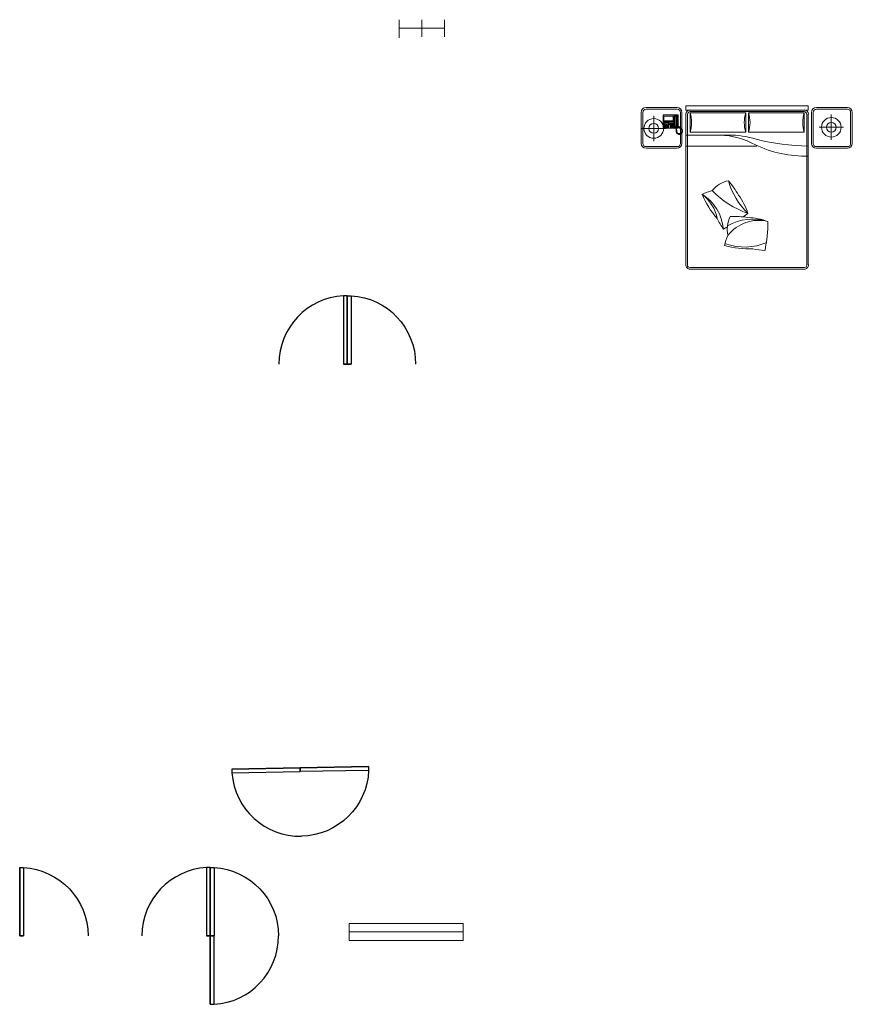
# Model space of a CAD drawing. Units: inches. Extents: x 907 to 2409, y 377 to 1163.
# Tile 9 of 9: x 1970 to 2409, y 443 to 961. Entities that reach past the tile are written whole.
import ezdxf

# ---------------------------------------------------------------- set-up
doc = ezdxf.new("R2010")
doc.units = ezdxf.units.IN
for name, color, linetype, lineweight in [('A-DOOR', 3, 'Continuous', 25), ('A-FURN', 8, 'Continuous', 18), ('A-GLAZ', 4, 'Continuous', 18)]:
    doc.layers.add(name, color=color, linetype=linetype, lineweight=lineweight)

# ---------------------------------------------------------------- blocks, each defined once
blk = doc.blocks.new('A$C356F0359')
for p, q in [((0.44, 1.98), (0.06, 1.98)), ((0.44, 1.96), (0.06, 1.96)), ((0.549, 2), (2.049, 2)), ((0.549, 1.949), (0.549, 2)), ((2.049, 1.949), (0.549, 1.949)), ((2.049, 1.949), (2.049, 2)), ((2.528, 1.98), (2.148, 1.98)), ((2.528, 1.96), (2.148, 1.96)), ((0, 1.92), (0, 1.54)), ((0.02, 1.92), (0.02, 1.54)), ((0.154, 1.568), (0.154, 1.878)), ((0.272, 1.888), (0.27, 1.886)), ((0.27, 1.886), (0.27, 1.728)), ((0.272, 1.888), (0.453, 1.888)), ((0.391, 1.875), (0.277, 1.875)), ((0.277, 1.875), (0.277, 1.815)), ((0.277, 1.815), (0.391, 1.815)), ((0.391, 1.812), (0.282, 1.812)), ((0.282, 1.812), (0.282, 1.801)), ((0.291, 1.812), (0.291, 1.801)), ((0.3, 1.812), (0.3, 1.801)), ((0.309, 1.812), (0.309, 1.801)), ((0.318, 1.812), (0.318, 1.801)), ((0.327, 1.812), (0.327, 1.801)), ((0.336, 1.812), (0.336, 1.801)), ((0.391, 1.815), (0.391, 1.875)), ((0.391, 1.801), (0.391, 1.812)), ((0.402, 1.879), (0.406, 1.884)), ((0.402, 1.74), (0.402, 1.879)), ((0.406, 1.881), (0.405, 1.876)), ((0.405, 1.876), (0.415, 1.866)), ((0.405, 1.876), (0.405, 1.846)), ((0.405, 1.846), (0.407, 1.84)), ((0.406, 1.884), (0.44, 1.884)), ((0.411, 1.883), (0.406, 1.881)), ((0.407, 1.84), (0.411, 1.834)), ((0.411, 1.883), (0.438, 1.883)), ((0.416, 1.868), (0.411, 1.883)), ((0.411, 1.834), (0.412, 1.826)), ((0.412, 1.826), (0.412, 1.815)), ((0.412, 1.793), (0.412, 1.815)), ((0.415, 1.866), (0.416, 1.868)), ((0.415, 1.815), (0.415, 1.866)), ((0.415, 1.815), (0.415, 1.753)), ((0.432, 1.868), (0.416, 1.868)), ((0.432, 1.868), (0.438, 1.883)), ((0.434, 1.866), (0.432, 1.868)), ((0.444, 1.876), (0.434, 1.866)), ((0.434, 1.815), (0.434, 1.866)), ((0.434, 1.815), (0.434, 1.753)), ((0.438, 1.834), (0.437, 1.826)), ((0.437, 1.826), (0.437, 1.815)), ((0.437, 1.793), (0.437, 1.815)), ((0.438, 1.883), (0.443, 1.881)), ((0.442, 1.84), (0.438, 1.834)), ((0.44, 1.884), (0.446, 1.879)), ((0.444, 1.846), (0.442, 1.84)), ((0.443, 1.881), (0.444, 1.876)), ((0.444, 1.876), (0.444, 1.846)), ((0.446, 1.879), (0.446, 1.742)), ((0.453, 1.888), (0.455, 1.886)), ((0.455, 1.886), (0.455, 1.728)), ((0.48, 1.54), (0.48, 1.92)), ((0.5, 1.54), (0.5, 1.92)), ((0.549, 1.898), (0.549, 0.051)), ((0.569, 1.898), (0.569, 0.051)), ((1.998, 1.929), (0.6, 1.929)), ((2.029, 0.051), (2.029, 1.898)), ((2.049, 0.051), (2.049, 1.898)), ((2.088, 1.92), (2.088, 1.54)), ((2.108, 1.92), (2.108, 1.54)), ((2.331, 1.582), (2.331, 1.892)), ((2.568, 1.54), (2.568, 1.92)), ((2.588, 1.54), (2.588, 1.92)), ((0.305, 1.723), (0.005, 1.723)), ((0.27, 1.728), (0.272, 1.726)), ((0.424, 1.726), (0.272, 1.726)), ((0.277, 1.788), (0.277, 1.768)), ((0.344, 1.788), (0.277, 1.788)), ((0.277, 1.768), (0.344, 1.768)), ((0.278, 1.762), (0.278, 1.758)), ((0.29, 1.762), (0.278, 1.762)), ((0.278, 1.758), (0.29, 1.758)), ((0.278, 1.745), (0.29, 1.745)), ((0.278, 1.738), (0.278, 1.745)), ((0.29, 1.738), (0.278, 1.738)), ((0.282, 1.801), (0.391, 1.801)), ((0.288, 1.786), (0.288, 1.783)), ((0.292, 1.786), (0.288, 1.786)), ((0.288, 1.783), (0.292, 1.783)), ((0.292, 1.774), (0.288, 1.774)), ((0.288, 1.774), (0.288, 1.77)), ((0.288, 1.77), (0.292, 1.77)), ((0.29, 1.758), (0.29, 1.762)), ((0.29, 1.745), (0.29, 1.738)), ((0.292, 1.783), (0.292, 1.786)), ((0.292, 1.77), (0.292, 1.774)), ((0.294, 1.762), (0.294, 1.758)), ((0.306, 1.762), (0.294, 1.762)), ((0.294, 1.758), (0.306, 1.758)), ((0.294, 1.745), (0.306, 1.745)), ((0.294, 1.738), (0.294, 1.745)), ((0.306, 1.738), (0.294, 1.738)), ((0.306, 1.758), (0.306, 1.762)), ((0.306, 1.745), (0.306, 1.738)), ((0.312, 1.786), (0.309, 1.786)), ((0.309, 1.786), (0.309, 1.783)), ((0.309, 1.783), (0.312, 1.783)), ((0.312, 1.774), (0.309, 1.774)), ((0.309, 1.774), (0.309, 1.77)), ((0.309, 1.77), (0.312, 1.77)), ((0.31, 1.762), (0.31, 1.758)), ((0.322, 1.762), (0.31, 1.762)), ((0.31, 1.758), (0.322, 1.758)), ((0.31, 1.745), (0.322, 1.745)), ((0.31, 1.738), (0.31, 1.745)), ((0.322, 1.738), (0.31, 1.738)), ((0.312, 1.783), (0.312, 1.786)), ((0.312, 1.77), (0.312, 1.774)), ((0.322, 1.758), (0.322, 1.762)), ((0.322, 1.745), (0.322, 1.738)), ((0.338, 1.762), (0.326, 1.762)), ((0.326, 1.762), (0.326, 1.758)), ((0.326, 1.758), (0.338, 1.758)), ((0.326, 1.738), (0.326, 1.745)), ((0.326, 1.745), (0.338, 1.745)), ((0.338, 1.738), (0.326, 1.738)), ((0.333, 1.786), (0.33, 1.786)), ((0.33, 1.786), (0.33, 1.783)), ((0.33, 1.783), (0.333, 1.783)), ((0.333, 1.774), (0.33, 1.774)), ((0.33, 1.774), (0.33, 1.77)), ((0.33, 1.77), (0.333, 1.77)), ((0.333, 1.783), (0.333, 1.786)), ((0.333, 1.77), (0.333, 1.774)), ((0.338, 1.758), (0.338, 1.762)), ((0.338, 1.745), (0.338, 1.738)), ((0.344, 1.768), (0.344, 1.788)), ((0.355, 1.776), (0.355, 1.783)), ((0.355, 1.783), (0.364, 1.783)), ((0.364, 1.776), (0.355, 1.776)), ((0.355, 1.763), (0.355, 1.77)), ((0.355, 1.77), (0.364, 1.77)), ((0.364, 1.763), (0.355, 1.763)), ((0.355, 1.756), (0.364, 1.756)), ((0.355, 1.75), (0.355, 1.756)), ((0.364, 1.75), (0.355, 1.75)), ((0.355, 1.737), (0.355, 1.744)), ((0.355, 1.744), (0.364, 1.744)), ((0.364, 1.737), (0.355, 1.737)), ((0.364, 1.783), (0.364, 1.776)), ((0.364, 1.77), (0.364, 1.763)), ((0.364, 1.756), (0.364, 1.75)), ((0.364, 1.744), (0.364, 1.737)), ((0.368, 1.783), (0.378, 1.783)), ((0.368, 1.776), (0.368, 1.783)), ((0.378, 1.776), (0.368, 1.776)), ((0.368, 1.763), (0.368, 1.77)), ((0.368, 1.77), (0.378, 1.77)), ((0.378, 1.763), (0.368, 1.763)), ((0.368, 1.756), (0.378, 1.756)), ((0.368, 1.75), (0.368, 1.756)), ((0.378, 1.75), (0.368, 1.75)), ((0.368, 1.737), (0.368, 1.744)), ((0.368, 1.744), (0.378, 1.744)), ((0.378, 1.737), (0.368, 1.737)), ((0.378, 1.783), (0.378, 1.776)), ((0.378, 1.77), (0.378, 1.763)), ((0.378, 1.756), (0.378, 1.75)), ((0.378, 1.744), (0.378, 1.737)), ((0.382, 1.776), (0.382, 1.783)), ((0.382, 1.783), (0.391, 1.783)), ((0.391, 1.776), (0.382, 1.776)), ((0.382, 1.763), (0.382, 1.77)), ((0.382, 1.77), (0.391, 1.77)), ((0.391, 1.763), (0.382, 1.763)), ((0.382, 1.758), (0.391, 1.758)), ((0.382, 1.751), (0.382, 1.758)), ((0.391, 1.751), (0.382, 1.751)), ((0.382, 1.744), (0.391, 1.744)), ((0.382, 1.737), (0.382, 1.744)), ((0.391, 1.737), (0.382, 1.737)), ((0.391, 1.783), (0.391, 1.776)), ((0.391, 1.77), (0.391, 1.763)), ((0.391, 1.758), (0.391, 1.751)), ((0.391, 1.744), (0.391, 1.737)), ((0.407, 1.735), (0.402, 1.74)), ((0.405, 1.774), (0.407, 1.779)), ((0.405, 1.743), (0.405, 1.774)), ((0.405, 1.743), (0.415, 1.753)), ((0.406, 1.738), (0.405, 1.743)), ((0.411, 1.736), (0.406, 1.738)), ((0.407, 1.779), (0.411, 1.785)), ((0.423, 1.735), (0.407, 1.735)), ((0.411, 1.785), (0.412, 1.793)), ((0.416, 1.751), (0.411, 1.736)), ((0.411, 1.736), (0.423, 1.736)), ((0.415, 1.753), (0.416, 1.751)), ((0.432, 1.751), (0.416, 1.751)), ((0.423, 1.739), (0.423, 1.729)), ((0.427, 1.739), (0.423, 1.739)), ((0.423, 1.729), (0.426, 1.718)), ((0.426, 1.718), (0.429, 1.707)), ((0.427, 1.73), (0.427, 1.739)), ((0.427, 1.736), (0.438, 1.736)), ((0.44, 1.735), (0.427, 1.735)), ((0.429, 1.723), (0.427, 1.73)), ((0.43, 1.7), (0.427, 1.697)), ((0.427, 1.697), (0.427, 1.691)), ((0.427, 1.691), (0.433, 1.69)), ((0.433, 1.69), (0.427, 1.686)), ((0.453, 1.726), (0.428, 1.726)), ((0.432, 1.712), (0.429, 1.723)), ((0.429, 1.707), (0.429, 1.701)), ((0.429, 1.701), (0.43, 1.7)), ((0.434, 1.753), (0.432, 1.751)), ((0.432, 1.751), (0.438, 1.736)), ((0.433, 1.706), (0.432, 1.712)), ((0.432, 1.7), (0.433, 1.706)), ((0.436, 1.697), (0.432, 1.7)), ((0.444, 1.743), (0.434, 1.753)), ((0.436, 1.692), (0.436, 1.697)), ((0.437, 1.677), (0.436, 1.692)), ((0.438, 1.785), (0.437, 1.793)), ((0.442, 1.779), (0.438, 1.785)), ((0.438, 1.736), (0.443, 1.738)), ((0.446, 1.742), (0.44, 1.735)), ((0.444, 1.774), (0.442, 1.779)), ((0.443, 1.738), (0.444, 1.743)), ((0.444, 1.743), (0.444, 1.774)), ((0.455, 1.728), (0.453, 1.726)), ((0.462, 1.746), (0.455, 1.748)), ((0.455, 1.744), (0.46, 1.742)), ((0.46, 1.742), (0.465, 1.739)), ((0.465, 1.743), (0.462, 1.746)), ((0.468, 1.74), (0.465, 1.743)), ((0.465, 1.739), (0.466, 1.737)), ((0.466, 1.737), (0.469, 1.737)), ((0.469, 1.737), (0.466, 1.735)), ((0.466, 1.735), (0.475, 1.727)), ((0.472, 1.742), (0.468, 1.74)), ((0.474, 1.74), (0.472, 1.742)), ((0.472, 1.737), (0.474, 1.74)), ((0.475, 1.739), (0.472, 1.737)), ((0.478, 1.736), (0.475, 1.739)), ((0.475, 1.727), (0.491, 1.714)), ((0.476, 1.729), (0.478, 1.736)), ((0.482, 1.732), (0.476, 1.729)), ((0.487, 1.727), (0.482, 1.732)), ((0.486, 1.72), (0.487, 1.727)), ((0.491, 1.723), (0.486, 1.72)), ((0.496, 1.718), (0.491, 1.723)), ((0.491, 1.713), (0.498, 1.692)), ((0.494, 1.713), (0.496, 1.718)), ((0.501, 1.714), (0.494, 1.713)), ((0.498, 1.692), (0.495, 1.674)), ((0.496, 1.705), (0.503, 1.707)), ((0.504, 1.705), (0.496, 1.705)), ((0.503, 1.707), (0.501, 1.714)), ((0.501, 1.695), (0.505, 1.7)), ((0.507, 1.695), (0.501, 1.695)), ((0.505, 1.7), (0.504, 1.705)), ((0.508, 1.689), (0.507, 1.695)), ((2.482, 1.737), (2.182, 1.737)), ((0.427, 1.686), (0.427, 1.68)), ((0.427, 1.68), (0.435, 1.679)), ((0.435, 1.679), (0.428, 1.674)), ((0.428, 1.674), (0.431, 1.669)), ((0.431, 1.669), (0.438, 1.67)), ((0.438, 1.67), (0.435, 1.664)), ((0.435, 1.664), (0.438, 1.66)), ((0.445, 1.666), (0.437, 1.677)), ((0.438, 1.66), (0.444, 1.664)), ((0.444, 1.664), (0.443, 1.657)), ((0.443, 1.657), (0.447, 1.655)), ((0.458, 1.66), (0.445, 1.666)), ((0.447, 1.655), (0.453, 1.659)), ((0.453, 1.659), (0.452, 1.652)), ((0.452, 1.652), (0.457, 1.65)), ((0.457, 1.65), (0.46, 1.657)), ((0.472, 1.659), (0.458, 1.66)), ((0.46, 1.657), (0.463, 1.65)), ((0.463, 1.65), (0.467, 1.65)), ((0.467, 1.65), (0.468, 1.657)), ((0.468, 1.657), (0.471, 1.649)), ((0.471, 1.649), (0.475, 1.65)), ((0.485, 1.664), (0.472, 1.659)), ((0.475, 1.65), (0.475, 1.657)), ((0.475, 1.657), (0.481, 1.652)), ((0.481, 1.652), (0.484, 1.654)), ((0.484, 1.654), (0.484, 1.661)), ((0.484, 1.661), (0.488, 1.655)), ((0.495, 1.674), (0.485, 1.664)), ((0.488, 1.655), (0.492, 1.658)), ((0.492, 1.658), (0.489, 1.664)), ((0.489, 1.664), (0.496, 1.661)), ((0.496, 1.67), (0.502, 1.668)), ((0.499, 1.664), (0.496, 1.67)), ((0.496, 1.661), (0.499, 1.664)), ((0.504, 1.673), (0.499, 1.679)), ((0.499, 1.679), (0.506, 1.679)), ((0.501, 1.687), (0.508, 1.689)), ((0.507, 1.684), (0.501, 1.687)), ((0.502, 1.668), (0.504, 1.673)), ((0.506, 1.679), (0.507, 1.684)), ((0.06, 1.5), (0.44, 1.5)), ((0.06, 1.48), (0.44, 1.48)), ((2.148, 1.5), (2.528, 1.5)), ((2.148, 1.48), (2.528, 1.48)), ((0.6, 0.02), (1.998, 0.02)), ((0.6, 0), (1.998, 0))]:
    blk.add_line(p, q)
at = {"linetype": 'ByBlock'}
for p, q in [((0.6, 1.915), (1.282, 1.915)), ((0.6, 1.676), (0.6, 1.915)), ((1.282, 1.915), (1.282, 1.676)), ((1.316, 1.915), (1.998, 1.915)), ((1.316, 1.676), (1.316, 1.915)), ((1.998, 1.915), (1.998, 1.676)), ((1.069, 1.642), (0.549, 1.642)), ((1.282, 1.676), (0.6, 1.676)), ((1.998, 1.676), (1.316, 1.676)), ((1.418, 1.505), (0.549, 1.505))]:
    blk.add_line(p, q, dxfattribs=at)
for centre in [(0.154, 1.723), (2.331, 1.737)]:
    blk.add_circle(centre, 0.12, dxfattribs=at)
for centre in [(0.154, 1.723), (2.331, 1.737)]:
    blk.add_circle(centre, 0.06)
for centre, radius, start, end in [((0.06, 1.92), 0.06, 90, 180), ((0.06, 1.92), 0.04, 90, 180), ((0.44, 1.92), 0.06, 0, 90), ((0.44, 1.92), 0.04, 0, 90), ((0.6, 1.898), 0.0512, 90, 180), ((1.998, 1.898), 0.0512, 0, 90), ((2.148, 1.92), 0.06, 90, 180), ((2.148, 1.92), 0.04, 90, 180), ((2.528, 1.92), 0.06, 0, 90), ((2.528, 1.92), 0.04, 0, 90), ((0.6, 1.898), 0.0312, 90, 180), ((1.998, 1.898), 0.0312, 0, 90), ((0.06, 1.54), 0.06, 180, 270), ((0.06, 1.54), 0.04, 180, 270), ((0.44, 1.54), 0.04, 270, 0), ((0.44, 1.54), 0.06, 270, 0), ((2.148, 1.54), 0.06, 180, 270), ((2.148, 1.54), 0.04, 180, 270), ((2.528, 1.54), 0.06, 270, 0), ((2.528, 1.54), 0.04, 270, 0), ((1.147, 0.733), 0.358, 102.4782, 140.4625), ((1.909, 1.312), 0.87, 195.336, 226.4193), ((0.325, 0.433), 0.988, 28.4971, 41.0566), ((0.997, 0.427), 0.548, 103.2034, 117.0362), ((0.445, 0.437), 0.566, 5.3391, 57.6895), ((0.452, 0.527), 0.488, 10.6986, 52.6864), ((1.819, 1.372), 1.165, 203.0642, 220.3209), ((1.653, 1.706), 1.08, 223.6306, 251.4288), ((0.562, 0.434), 0.787, 18.3527, 36.6851), ((1.595, 0.931), 0.734, 205.259, 216.9351), ((1.413, 0.487), 0.358, 154.0418, 192.0262), ((1.364, 0.004), 0.608, 71.81, 120.1351), ((1.137, -0.343), 0.988, 80.0607, 92.6202), ((-0.021, 2.432), 2.198, 305.2966, 307.2418), ((1.284, -0.157), 0.787, 69.9163, 88.2487), ((-0.021, 2.432), 2.198, 297.9248, 299.3793), ((1.44, 0.119), 0.477, 76.1849, 142.0017), ((-0.643, 0.628), 2.198, 349.4884, 358.8054), ((1.559, 0.179), 0.548, 154.767, 168.5998), ((1.331, 1.411), 1.165, 254.6278, 271.8845), ((1.265, 0.958), 0.689, 250.2936, 293.6414), ((1.537, 0.961), 0.734, 256.8226, 268.4988), ((0.594, 0.045), 0.0458, 172.7599, 277.2401), ((0.594, 0.045), 0.0258, 172.7599, 277.2401), ((2.004, 0.045), 0.0458, 262.7599, 7.2401), ((2.004, 0.045), 0.0258, 262.7599, 7.2401)]:
    blk.add_arc(centre, radius, start, end)
for centre, radius, start, end in [((0.191, 1.795), 0.427, 343.7398, 16.2602), ((1.691, 1.795), 0.427, 163.7398, 196.2602), ((0.907, 1.795), 0.427, 343.7398, 16.2602), ((2.407, 1.795), 0.427, 163.7398, 196.2602), ((0.93, 0.657), 0.985, 61.4328, 88.1261), ((1.083, 0.571), 1.071, 72.1966, 90.7418), ((2.137, 4.6), 3.096, 256.4201, 268.3789), ((2.006, 2.774), 1.39, 244.2427, 271.7984)]:
    blk.add_arc(centre, radius, start, end, dxfattribs=at)
blk = doc.blocks.new('DOOR-36IN')
for p, q in [((36, 36), (36, 0)), ((36, 0), (34, 0)), ((36, 0), (34, 0))]:
    blk.add_line(p, q)
blk.add_lwpolyline([(36, 36), (34, 36), (34, 0), (36, 0)], close=True)
blk.add_arc((36.06, 0), 36.06, 93.2732, 180)
blk = doc.blocks.new('WIN-24IN')
for p, q in [((0.53, 23.99), (0, 23.99)), ((9.53, 24), (0.53, 24)), ((5.03, 0), (5.03, 24)), ((9.53, 12), (0.53, 12)), ((9.53, 0), (0.53, 0))]:
    blk.add_line(p, q)
blk = doc.blocks.new('WIN-60IN')
for p, q in [((0, 9), (0, 0)), ((0, 4.5), (60, 4.5)), ((0, 0), (60, 0))]:
    blk.add_line(p, q)
blk.add_lwpolyline([(0, 9), (60, 9), (60, 0), (0, 0)], close=True)

msp = doc.modelspace()

# ---------------------------------------------------------------- block references
at = {"layer": 'A-DOOR'}
for p in [(2106.9071, 779.6791), (2034.735, 478.592)]:
    msp.add_blockref('DOOR-36IN', p, dxfattribs=at)
at = {"layer": 'A-DOOR', "extrusion": (0, 0, -1), "zscale": -1}
for p in [(-2178.9071, 779.6791), (-2006.392, 478.592), (-2106.735, 478.592)]:
    msp.add_blockref('DOOR-36IN', p, dxfattribs=at)
at = {"layer": 'A-DOOR'}
for p, rotation in [((2118.8034, 531.0979), 91.08740474419417), ((2106.735, 478.592), 180)]:
    msp.add_blockref('DOOR-36IN', p, dxfattribs=dict(at, rotation=rotation))
at = {"layer": 'A-DOOR', "extrusion": (0, 0, -1), "zscale": -1, "rotation": 88.91259525590984}
msp.add_blockref('DOOR-36IN', (-2118.8034, 531.0979), dxfattribs=at)
at = {"layer": 'A-FURN', "xscale": 42.95257138859579, "yscale": 42.95257138859579, "zscale": 42.95257138859579}
msp.add_blockref('A$C356F0359', (2297.7069, 829.7336), dxfattribs=at)
at = {"layer": 'A-GLAZ', "rotation": 90.00000000000156}
msp.add_blockref('WIN-24IN', (2194.1617, 951.4663), dxfattribs=at)
at = {"layer": 'A-GLAZ'}
msp.add_blockref('WIN-60IN', (2143.871, 476.187), dxfattribs=at)

doc.saveas('drawing.dxf')
